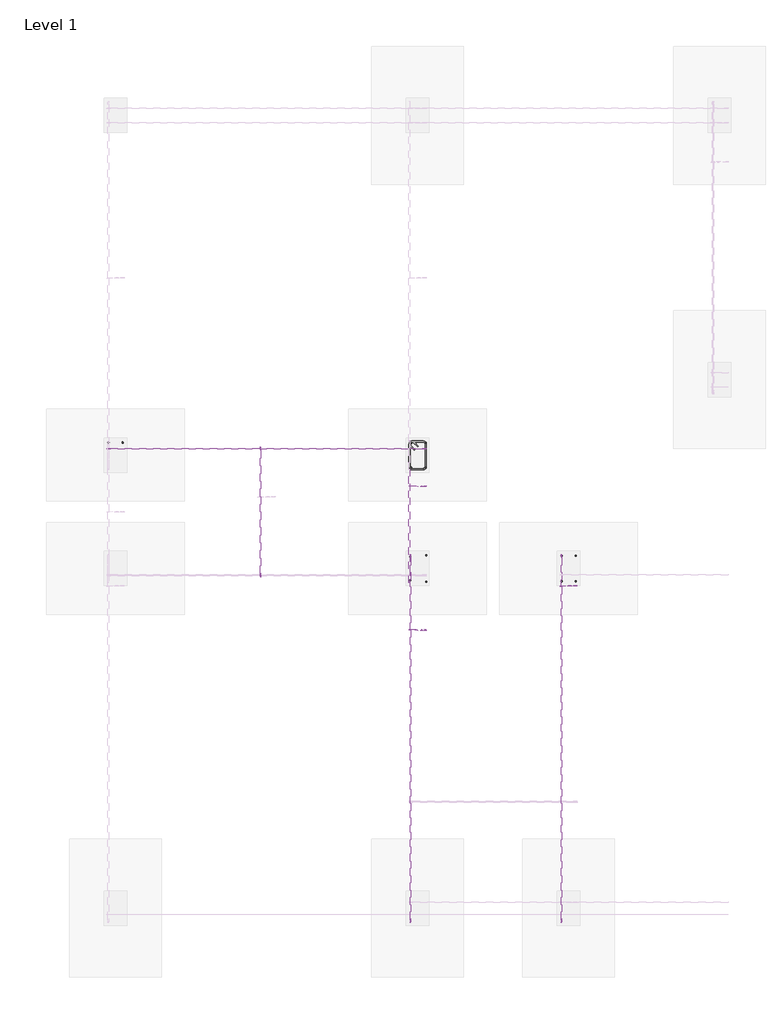
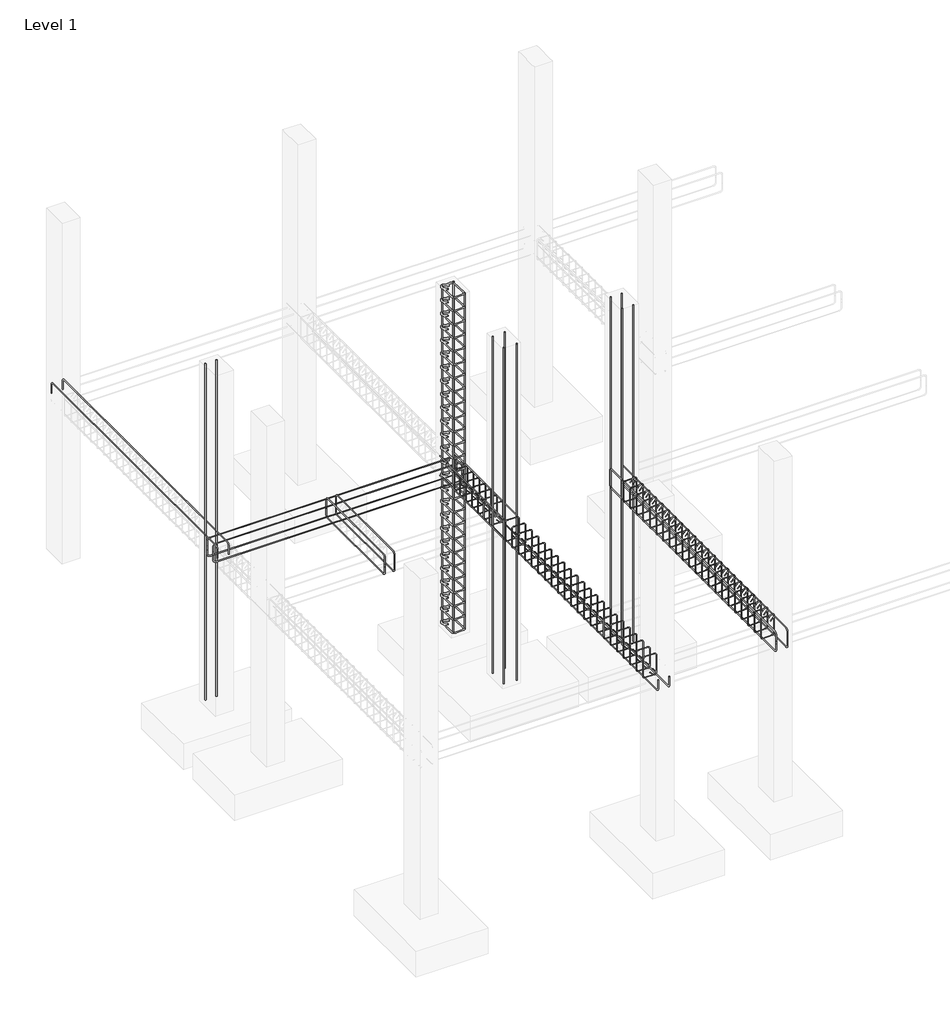
# One storey, part 3 of 5: 21 reinforcing bars.
"""IFC4 building model written with IfcOpenShell, lengths in millimetres."""

from ifc_helpers import new_model, si_unit, point, frame, origin, place, context, project, spatial, polyline, circle_curve, trimmed, segment, composite_curve, source, transform, mapped, element, save
from ifc_brep_helpers import swept_disk

model = new_model("IFC4")

# Units and contexts
model_context = context("Model", 3, world=origin())
ifc_project = project(units=[si_unit("LENGTHUNIT", "METRE", prefix="MILLI")], contexts=[model_context])

# Site, building, storey
site = spatial("IfcSite", under=ifc_project)
building = spatial("IfcBuilding", under=site)
storey = spatial("IfcBuildingStorey", under=building, Name="Level 1", Elevation=0.0)

# Reinforcing bars
placement = place(None, origin())
reinforcing_bar_shape = source(origin(), model_context, "Body", "SolidModel", [
    swept_disk(composite_curve([segment(polyline([(-15212.455746, 8562.3577522, 2793.8967919), (-15212.455746, 8562.3577522, 2946.2967919)]), True, "CONTINUOUS"), segment(trimmed(circle_curve(frame((-15212.455746, 8518.2887522, 2946.2967919), z_axis=(1.0, 0.0, 0.0), x_axis=(0.0, 44.068999999999505, 0.0)), 44.069), [point((-15212.455746, 8562.3577522, 2946.2967919))], [point((-15212.455746, 8518.2887522, 2990.3657919))], True, "CARTESIAN"), True, "CONTINUOUS"), segment(polyline([(-15212.455746, 8518.2887522, 2990.3657919), (-15212.455746, 3737.3647522, 2990.3657919)]), True, "CONTINUOUS"), segment(trimmed(circle_curve(frame((-15212.455746, 3737.3647522, 2946.2967919), z_axis=(1.0, 0.0, 0.0), x_axis=(0.0, 0.0, 44.069000000000415)), 44.069), [point((-15212.455746, 3737.3647522, 2990.3657919))], [point((-15212.455746, 3693.2957522, 2946.2967919))], True, "CARTESIAN"), True, "CONTINUOUS"), segment(polyline([(-15212.455746, 3693.2957522, 2946.2967919), (-15212.455746, 3693.2957522, 2793.8967919)]), True, "CONTINUOUS")], self_intersect=False), 5.969),
])
element("IfcReinforcingBar", 1, at=placement, inside=storey, context=model_context, shape_type="MappedRepresentation", body=[
    mapped(reinforcing_bar_shape, transform((0.0, 0.0, 0.0), x_axis=(1.0, 0.0, 0.0), y_axis=(0.0, 1.0, 0.0), z_axis=(0.0, 0.0, 1.0))),
    mapped(reinforcing_bar_shape, transform((-189.5315837, 0.0, 0.0), x_axis=(1.0, 0.0, 0.0), y_axis=(0.0, 1.0, 0.0), z_axis=(0.0, 0.0, 1.0))),
])
reinforcing_bar_2_shape = source(origin(), model_context, "Body", "SolidModel", [
    swept_disk(composite_curve([segment(polyline([(-15213.892587, 4047.3557031, 38.1), (-15213.892587, 4047.3557031, 6057.9)]), True, "CONTINUOUS")], self_intersect=False), 8.001),
])
element("IfcReinforcingBar", 2, at=placement, inside=storey, context=model_context, shape_type="MappedRepresentation", body=[
    mapped(reinforcing_bar_2_shape, transform((0.0, 0.0, 0.0), x_axis=(1.0, 0.0, 0.0), y_axis=(0.0, 1.0, 0.0), z_axis=(0.0, 0.0, 1.0))),
    mapped(reinforcing_bar_2_shape, transform((-186.6579018, 0.0, 0.0), x_axis=(1.0, 0.0, 0.0), y_axis=(0.0, 1.0, 0.0), z_axis=(0.0, 0.0, 1.0))),
])
reinforcing_bar_3_shape = source(origin(), model_context, "Body", "SolidModel", [
    swept_disk(composite_curve([segment(polyline([(-13226.1955379, 3986.1577522, 2799.588), (-13226.1955379, 3986.1577522, 2951.988)]), True, "CONTINUOUS"), segment(trimmed(circle_curve(frame((-13226.1955379, 3942.0887522, 2951.988), z_axis=(1.0, 0.0, 0.0), x_axis=(0.0, 44.06899999999996, 0.0)), 44.069), [point((-13226.1955379, 3986.1577522, 2951.988))], [point((-13226.1955379, 3942.0887522, 2996.057))], True, "CARTESIAN"), True, "CONTINUOUS"), segment(polyline([(-13226.1955379, 3942.0887522, 2996.057), (-13226.1955379, 2313.5647522, 2996.057)]), True, "CONTINUOUS"), segment(trimmed(circle_curve(frame((-13226.1955379, 2313.5647522, 2951.988), z_axis=(1.0, 0.0, 0.0), x_axis=(0.0, 0.0, 44.06899999999996)), 44.069), [point((-13226.1955379, 2313.5647522, 2996.057))], [point((-13226.1955379, 2269.4957522, 2951.988))], True, "CARTESIAN"), True, "CONTINUOUS"), segment(polyline([(-13226.1955379, 2269.4957522, 2951.988), (-13226.1955379, 2269.4957522, 2799.588)]), True, "CONTINUOUS")], self_intersect=False), 5.969),
])
element("IfcReinforcingBar", 3, at=placement, inside=storey, context=model_context, shape_type="MappedRepresentation", body=[
    mapped(reinforcing_bar_3_shape, transform((0.0, 0.0, 0.0), x_axis=(1.0, 0.0, 0.0), y_axis=(0.0, 1.0, 0.0), z_axis=(0.0, 0.0, 1.0))),
    mapped(reinforcing_bar_3_shape, transform((-162.052, 0.0, 0.0), x_axis=(1.0, 0.0, 0.0), y_axis=(0.0, 1.0, 0.0), z_axis=(0.0, 0.0, 1.0))),
])
reinforcing_bar_4_shape = source(origin(), model_context, "Body", "SolidModel", [
    swept_disk(composite_curve([segment(polyline([(-13388.2475379, 2269.4957522, 2839.212), (-13388.2475379, 2269.4957522, 2686.812)]), True, "CONTINUOUS"), segment(trimmed(circle_curve(frame((-13388.2475379, 2313.5647522, 2686.812), z_axis=(1.0, 0.0, 0.0), x_axis=(0.0, -44.06899999999996, 0.0)), 44.069), [point((-13388.2475379, 2269.4957522, 2686.812))], [point((-13388.2475379, 2313.5647522, 2642.743))], True, "CARTESIAN"), True, "CONTINUOUS"), segment(polyline([(-13388.2475379, 2313.5647522, 2642.743), (-13388.2475379, 3942.0887522, 2642.743)]), True, "CONTINUOUS"), segment(trimmed(circle_curve(frame((-13388.2475379, 3942.0887522, 2686.812), z_axis=(1.0, 0.0, 0.0), x_axis=(0.0, 0.0, -44.06899999999996)), 44.069), [point((-13388.2475379, 3942.0887522, 2642.743))], [point((-13388.2475379, 3986.1577522, 2686.812))], True, "CARTESIAN"), True, "CONTINUOUS"), segment(polyline([(-13388.2475379, 3986.1577522, 2686.812), (-13388.2475379, 3986.1577522, 2839.212)]), True, "CONTINUOUS")], self_intersect=False), 5.969),
])
element("IfcReinforcingBar", 4, at=placement, inside=storey, context=model_context, shape_type="MappedRepresentation", body=[
    mapped(reinforcing_bar_4_shape, transform((0.0, 0.0, 0.0), x_axis=(1.0, 0.0, 0.0), y_axis=(0.0, 1.0, 0.0), z_axis=(0.0, 0.0, 1.0))),
    mapped(reinforcing_bar_4_shape, transform((162.052, 0.0, 0.0), x_axis=(1.0, 0.0, 0.0), y_axis=(0.0, 1.0, 0.0), z_axis=(0.0, 0.0, 1.0))),
])
reinforcing_bar_5_shape = source(origin(), model_context, "Body", "SolidModel", [
    swept_disk(composite_curve([segment(polyline([(-15415.5525379, 3964.464544, 2785.7687919), (-15415.5525379, 3964.464544, 2938.1687919)]), True, "CONTINUOUS"), segment(trimmed(circle_curve(frame((-15371.4835379, 3964.464544, 2938.1687919), z_axis=(0.0, 1.0, 0.0), x_axis=(-44.068999999999505, 0.0, 0.0)), 44.069), [point((-15415.5525379, 3964.464544, 2938.1687919))], [point((-15371.4835379, 3964.464544, 2982.2377919))], True, "CARTESIAN"), True, "CONTINUOUS"), segment(polyline([(-15371.4835379, 3964.464544, 2982.2377919), (-11242.9595379, 3964.464544, 2982.2377919)]), True, "CONTINUOUS"), segment(trimmed(circle_curve(frame((-11242.9595379, 3964.464544, 2938.1687919), z_axis=(0.0, 1.0, 0.0), x_axis=(0.0, 0.0, 44.06899999999996)), 44.069), [point((-11242.9595379, 3964.464544, 2982.2377919))], [point((-11198.8905379, 3964.464544, 2938.1687919))], True, "CARTESIAN"), True, "CONTINUOUS"), segment(polyline([(-11198.8905379, 3964.464544, 2938.1687919), (-11198.8905379, 3964.464544, 2785.7687919)]), True, "CONTINUOUS")], self_intersect=False), 5.969),
])
element("IfcReinforcingBar", 5, at=placement, inside=storey, context=model_context, shape_type="MappedRepresentation", body=[
    mapped(reinforcing_bar_5_shape, transform((0.0, 0.0, 0.0), x_axis=(1.0, 0.0, 0.0), y_axis=(0.0, 1.0, 0.0), z_axis=(0.0, 0.0, 1.0))),
    mapped(reinforcing_bar_5_shape, transform((0.0, -173.2755837, 0.0), x_axis=(1.0, 0.0, 0.0), y_axis=(0.0, 1.0, 0.0), z_axis=(0.0, 0.0, 1.0))),
])
reinforcing_bar_6_shape = source(origin(), model_context, "Body", "SolidModel", [
    swept_disk(composite_curve([segment(polyline([(-11198.8905379, 3964.464544, 2853.0312081), (-11198.8905379, 3964.464544, 2700.6312081)]), True, "CONTINUOUS"), segment(trimmed(circle_curve(frame((-11242.9595379, 3964.464544, 2700.6312081), z_axis=(0.0, 1.0, 0.0), x_axis=(44.068999999999505, 0.0, 0.0)), 44.069), [point((-11198.8905379, 3964.464544, 2700.6312081))], [point((-11242.9595379, 3964.464544, 2656.5622081))], True, "CARTESIAN"), True, "CONTINUOUS"), segment(polyline([(-11242.9595379, 3964.464544, 2656.5622081), (-15371.4835379, 3964.464544, 2656.5622081)]), True, "CONTINUOUS"), segment(trimmed(circle_curve(frame((-15371.4835379, 3964.464544, 2700.6312081), z_axis=(0.0, 1.0, 0.0), x_axis=(0.0, 0.0, -44.06899999999996)), 44.069), [point((-15371.4835379, 3964.464544, 2656.5622081))], [point((-15415.5525379, 3964.464544, 2700.6312081))], True, "CARTESIAN"), True, "CONTINUOUS"), segment(polyline([(-15415.5525379, 3964.464544, 2700.6312081), (-15415.5525379, 3964.464544, 2853.0312081)]), True, "CONTINUOUS")], self_intersect=False), 5.969),
])
element("IfcReinforcingBar", 6, at=placement, inside=storey, context=model_context, shape_type="MappedRepresentation", body=[
    mapped(reinforcing_bar_6_shape, transform((0.0, 0.0, 0.0), x_axis=(1.0, 0.0, 0.0), y_axis=(0.0, 1.0, 0.0), z_axis=(0.0, 0.0, 1.0))),
    mapped(reinforcing_bar_6_shape, transform((0.0, -173.2755837, 0.0), x_axis=(1.0, 0.0, 0.0), y_axis=(0.0, 1.0, 0.0), z_axis=(0.0, 0.0, 1.0))),
])
reinforcing_bar_7_shape = source(origin(), model_context, "Body", "SolidModel", [
    swept_disk(composite_curve([segment(polyline([(-11392.4224888, 4039.2277031, 38.1), (-11392.4224888, 4039.2277031, 6057.9)]), True, "CONTINUOUS")], self_intersect=False), 8.001),
])
element("IfcReinforcingBar", 7, at=placement, inside=storey, context=model_context, shape_type="MappedRepresentation", body=[
    mapped(reinforcing_bar_7_shape, transform((0.0, 0.0, 0.0), x_axis=(1.0, 0.0, 0.0), y_axis=(0.0, 1.0, 0.0), z_axis=(0.0, 0.0, 1.0))),
    mapped(reinforcing_bar_7_shape, transform((0.0, -322.8019018, 0.0), x_axis=(1.0, 0.0, 0.0), y_axis=(0.0, 1.0, 0.0), z_axis=(0.0, 0.0, 1.0))),
])
reinforcing_bar_8_shape = source(origin(), model_context, "Body", "SolidModel", [
    swept_disk(composite_curve([segment(polyline([(-11200.9225379, 4044.3237522, 6057.9), (-11200.9225379, 4044.3237522, 38.1)]), True, "CONTINUOUS")], self_intersect=False), 8.001),
])
element("IfcReinforcingBar", 8, at=placement, inside=storey, context=model_context, shape_type="MappedRepresentation", body=[
    mapped(reinforcing_bar_8_shape, transform((0.0, 0.0, 0.0), x_axis=(1.0, 0.0, 0.0), y_axis=(0.0, 1.0, 0.0), z_axis=(0.0, 0.0, 1.0))),
    mapped(reinforcing_bar_8_shape, transform((0.0, -332.994, 0.0), x_axis=(1.0, 0.0, 0.0), y_axis=(0.0, 1.0, 0.0), z_axis=(0.0, 0.0, 1.0))),
])
reinforcing_bar_9_shape = source(origin(), model_context, "Body", "SolidModel", [
    swept_disk(composite_curve([segment(polyline([(-11301.6364658, 3995.6778273, 46.101), (-11356.5014643, 4050.5428258, 46.101)]), True, "CONTINUOUS"), segment(trimmed(circle_curve(frame((-11380.1195379, 4026.9247522, 46.101), z_axis=(0.0, 0.0, 1.0), x_axis=(23.61807360000057, 23.618073600000116, 0.0)), 33.401), [point((-11356.5014643, 4050.5428258, 46.101))], [point((-11413.5205379, 4026.9247522, 46.101))], True, "CARTESIAN"), True, "CONTINUOUS"), segment(polyline([(-11413.5205379, 4026.9247522, 46.101), (-11413.5205379, 3728.7287522, 46.101)]), True, "CONTINUOUS"), segment(trimmed(circle_curve(frame((-11380.1195379, 3728.7287522, 46.101), z_axis=(0.0, 0.0, 1.0), x_axis=(-33.40099999999984, 0.0, 0.0)), 33.401), [point((-11413.5205379, 3728.7287522, 46.101))], [point((-11380.1195379, 3695.3277522, 46.101))], True, "CARTESIAN"), True, "CONTINUOUS"), segment(polyline([(-11380.1195379, 3695.3277522, 46.101), (-11234.3235379, 3695.3277522, 46.101)]), True, "CONTINUOUS"), segment(trimmed(circle_curve(frame((-11234.3235379, 3728.696699, 44.6380608), z_axis=(0.0, 0.043799263856762964, 0.9990403517804503), x_axis=(0.0, -33.36894680000023, 1.462939200000001)), 33.401), [point((-11234.3235379, 3695.3277522, 46.101))], [point((-11200.9225379, 3728.696699, 44.6380608))], True, "CARTESIAN"), True, "CONTINUOUS"), segment(polyline([(-11200.9225379, 3728.696699, 44.6380608), (-11200.9225379, 4026.9568054, 31.5619392)]), True, "CONTINUOUS"), segment(trimmed(circle_curve(frame((-11234.3235379, 4026.9568054, 31.5619392), z_axis=(0.0, 0.043799263856762964, 0.9990403517804503), x_axis=(33.40099999999984, 0.0, 0.0)), 33.401), [point((-11200.9225379, 4026.9568054, 31.5619392))], [point((-11234.3235379, 4060.3257522, 30.099))], True, "CARTESIAN"), True, "CONTINUOUS"), segment(polyline([(-11234.3235379, 4060.3257522, 30.099), (-11380.1195379, 4060.3257522, 30.099)]), True, "CONTINUOUS"), segment(trimmed(circle_curve(frame((-11380.1195379, 4026.9247522, 30.099), z_axis=(0.0, 0.0, 1.0), x_axis=(0.0, 33.40099999999984, 0.0)), 33.401), [point((-11380.1195379, 4060.3257522, 30.099))], [point((-11403.7376115, 4003.3066786, 30.099))], True, "CARTESIAN"), True, "CONTINUOUS"), segment(polyline([(-11403.7376115, 4003.3066786, 30.099), (-11348.872613, 3948.4416801, 30.099)]), True, "CONTINUOUS")], self_intersect=False), 8.001),
])
element("IfcReinforcingBar", 9, at=placement, inside=storey, context=model_context, shape_type="MappedRepresentation", body=[
    mapped(reinforcing_bar_9_shape, transform((0.0, 0.0, 0.0), x_axis=(1.0, 0.0, 0.0), y_axis=(0.0, 1.0, 0.0), z_axis=(0.0, 0.0, 1.0))),
    mapped(reinforcing_bar_9_shape, transform((0.0, 0.0, 240.15192), x_axis=(1.0, 0.0, 0.0), y_axis=(0.0, 1.0, 0.0), z_axis=(0.0, 0.0, 1.0))),
    mapped(reinforcing_bar_9_shape, transform((0.0, 0.0, 480.30384), x_axis=(1.0, 0.0, 0.0), y_axis=(0.0, 1.0, 0.0), z_axis=(0.0, 0.0, 1.0))),
    mapped(reinforcing_bar_9_shape, transform((0.0, 0.0, 720.45576), x_axis=(1.0, 0.0, 0.0), y_axis=(0.0, 1.0, 0.0), z_axis=(0.0, 0.0, 1.0))),
    mapped(reinforcing_bar_9_shape, transform((0.0, 0.0, 960.60768), x_axis=(1.0, 0.0, 0.0), y_axis=(0.0, 1.0, 0.0), z_axis=(0.0, 0.0, 1.0))),
    mapped(reinforcing_bar_9_shape, transform((0.0, 0.0, 1200.7596), x_axis=(1.0, 0.0, 0.0), y_axis=(0.0, 1.0, 0.0), z_axis=(0.0, 0.0, 1.0))),
    mapped(reinforcing_bar_9_shape, transform((0.0, 0.0, 1440.91152), x_axis=(1.0, 0.0, 0.0), y_axis=(0.0, 1.0, 0.0), z_axis=(0.0, 0.0, 1.0))),
    mapped(reinforcing_bar_9_shape, transform((0.0, 0.0, 1681.06344), x_axis=(1.0, 0.0, 0.0), y_axis=(0.0, 1.0, 0.0), z_axis=(0.0, 0.0, 1.0))),
    mapped(reinforcing_bar_9_shape, transform((0.0, 0.0, 1921.21536), x_axis=(1.0, 0.0, 0.0), y_axis=(0.0, 1.0, 0.0), z_axis=(0.0, 0.0, 1.0))),
    mapped(reinforcing_bar_9_shape, transform((0.0, 0.0, 2161.36728), x_axis=(1.0, 0.0, 0.0), y_axis=(0.0, 1.0, 0.0), z_axis=(0.0, 0.0, 1.0))),
    mapped(reinforcing_bar_9_shape, transform((0.0, 0.0, 2401.5192), x_axis=(1.0, 0.0, 0.0), y_axis=(0.0, 1.0, 0.0), z_axis=(0.0, 0.0, 1.0))),
    mapped(reinforcing_bar_9_shape, transform((0.0, 0.0, 2641.67112), x_axis=(1.0, 0.0, 0.0), y_axis=(0.0, 1.0, 0.0), z_axis=(0.0, 0.0, 1.0))),
    mapped(reinforcing_bar_9_shape, transform((0.0, 0.0, 2881.82304), x_axis=(1.0, 0.0, 0.0), y_axis=(0.0, 1.0, 0.0), z_axis=(0.0, 0.0, 1.0))),
    mapped(reinforcing_bar_9_shape, transform((0.0, 0.0, 3121.97496), x_axis=(1.0, 0.0, 0.0), y_axis=(0.0, 1.0, 0.0), z_axis=(0.0, 0.0, 1.0))),
    mapped(reinforcing_bar_9_shape, transform((0.0, 0.0, 3362.12688), x_axis=(1.0, 0.0, 0.0), y_axis=(0.0, 1.0, 0.0), z_axis=(0.0, 0.0, 1.0))),
    mapped(reinforcing_bar_9_shape, transform((0.0, 0.0, 3602.2788), x_axis=(1.0, 0.0, 0.0), y_axis=(0.0, 1.0, 0.0), z_axis=(0.0, 0.0, 1.0))),
    mapped(reinforcing_bar_9_shape, transform((0.0, 0.0, 3842.43072), x_axis=(1.0, 0.0, 0.0), y_axis=(0.0, 1.0, 0.0), z_axis=(0.0, 0.0, 1.0))),
    mapped(reinforcing_bar_9_shape, transform((0.0, 0.0, 4082.58264), x_axis=(1.0, 0.0, 0.0), y_axis=(0.0, 1.0, 0.0), z_axis=(0.0, 0.0, 1.0))),
    mapped(reinforcing_bar_9_shape, transform((0.0, 0.0, 4322.73456), x_axis=(1.0, 0.0, 0.0), y_axis=(0.0, 1.0, 0.0), z_axis=(0.0, 0.0, 1.0))),
    mapped(reinforcing_bar_9_shape, transform((0.0, 0.0, 4562.88648), x_axis=(1.0, 0.0, 0.0), y_axis=(0.0, 1.0, 0.0), z_axis=(0.0, 0.0, 1.0))),
    mapped(reinforcing_bar_9_shape, transform((0.0, 0.0, 4803.0384), x_axis=(1.0, 0.0, 0.0), y_axis=(0.0, 1.0, 0.0), z_axis=(0.0, 0.0, 1.0))),
    mapped(reinforcing_bar_9_shape, transform((0.0, 0.0, 5043.19032), x_axis=(1.0, 0.0, 0.0), y_axis=(0.0, 1.0, 0.0), z_axis=(0.0, 0.0, 1.0))),
    mapped(reinforcing_bar_9_shape, transform((0.0, 0.0, 5283.34224), x_axis=(1.0, 0.0, 0.0), y_axis=(0.0, 1.0, 0.0), z_axis=(0.0, 0.0, 1.0))),
    mapped(reinforcing_bar_9_shape, transform((0.0, 0.0, 5523.49416), x_axis=(1.0, 0.0, 0.0), y_axis=(0.0, 1.0, 0.0), z_axis=(0.0, 0.0, 1.0))),
    mapped(reinforcing_bar_9_shape, transform((0.0, 0.0, 5763.64608), x_axis=(1.0, 0.0, 0.0), y_axis=(0.0, 1.0, 0.0), z_axis=(0.0, 0.0, 1.0))),
    mapped(reinforcing_bar_9_shape, transform((0.0, 0.0, 6003.798), x_axis=(1.0, 0.0, 0.0), y_axis=(0.0, 1.0, 0.0), z_axis=(0.0, 0.0, 1.0))),
])
reinforcing_bar_10_shape = source(origin(), model_context, "Body", "SolidModel", [
    swept_disk(composite_curve([segment(polyline([(-11192.9215379, 2203.2017522, 38.1), (-11192.9215379, 2203.2017522, 6057.9)]), True, "CONTINUOUS")], self_intersect=False), 8.001),
])
element("IfcReinforcingBar", 10, at=placement, inside=storey, context=model_context, shape_type="MappedRepresentation", body=[
    mapped(reinforcing_bar_10_shape, transform((0.0, 0.0, 0.0), x_axis=(1.0, 0.0, 0.0), y_axis=(0.0, 1.0, 0.0), z_axis=(0.0, 0.0, 1.0))),
    mapped(reinforcing_bar_10_shape, transform((0.0, 349.25, 0.0), x_axis=(1.0, 0.0, 0.0), y_axis=(0.0, 1.0, 0.0), z_axis=(0.0, 0.0, 1.0))),
])
reinforcing_bar_11_shape = source(origin(), model_context, "Body", "SolidModel", [
    swept_disk(composite_curve([segment(polyline([(-11405.6465379, 2535.0527522, 6057.9), (-11405.6465379, 2535.0527522, 38.1)]), True, "CONTINUOUS")], self_intersect=False), 8.001),
])
element("IfcReinforcingBar", 11, at=placement, inside=storey, context=model_context, shape_type="MappedRepresentation", body=[
    mapped(reinforcing_bar_11_shape, transform((0.0, 0.0, 0.0), x_axis=(1.0, 0.0, 0.0), y_axis=(0.0, 1.0, 0.0), z_axis=(0.0, 0.0, 1.0))),
    mapped(reinforcing_bar_11_shape, transform((0.0, -314.452, 0.0), x_axis=(1.0, 0.0, 0.0), y_axis=(0.0, 1.0, 0.0), z_axis=(0.0, 0.0, 1.0))),
])
reinforcing_bar_12_shape = source(origin(), model_context, "Body", "SolidModel", [
    swept_disk(composite_curve([segment(polyline([(-11198.8905379, 4068.3267522, 2996.057), (-11198.8905379, 2187.3267522, 2996.057)]), True, "CONTINUOUS")], self_intersect=False), 5.969),
])
element("IfcReinforcingBar", 12, at=placement, inside=storey, context=model_context, shape_type="MappedRepresentation", body=[
    mapped(reinforcing_bar_12_shape, transform((0.0, 0.0, 0.0), x_axis=(1.0, 0.0, 0.0), y_axis=(0.0, 1.0, 0.0), z_axis=(0.0, 0.0, 1.0))),
    mapped(reinforcing_bar_12_shape, transform((-216.662, 0.0, 0.0), x_axis=(1.0, 0.0, 0.0), y_axis=(0.0, 1.0, 0.0), z_axis=(0.0, 0.0, 1.0))),
])
reinforcing_bar_13_shape = source(origin(), model_context, "Body", "SolidModel", [
    swept_disk(composite_curve([segment(polyline([(-11212.455746, 2187.3267522, 2648.4342081), (-11212.455746, 4068.3267522, 2648.4342081)]), True, "CONTINUOUS")], self_intersect=False), 5.969),
])
element("IfcReinforcingBar", 13, at=placement, inside=storey, context=model_context, shape_type="MappedRepresentation", body=[
    mapped(reinforcing_bar_13_shape, transform((0.0, 0.0, 0.0), x_axis=(1.0, 0.0, 0.0), y_axis=(0.0, 1.0, 0.0), z_axis=(0.0, 0.0, 1.0))),
    mapped(reinforcing_bar_13_shape, transform((-203.0967919, 0.0, 0.0), x_axis=(1.0, 0.0, 0.0), y_axis=(0.0, 1.0, 0.0), z_axis=(0.0, 0.0, 1.0))),
])
reinforcing_bar_14_shape = source(origin(), model_context, "Body", "SolidModel", [
    swept_disk(composite_curve([segment(polyline([(-11212.455746, -2306.7042478, 2844.9032081), (-11212.455746, -2306.7042478, 2692.5032081)]), True, "CONTINUOUS"), segment(trimmed(circle_curve(frame((-11212.455746, -2262.6352478, 2692.5032081), z_axis=(1.0, 0.0, 0.0), x_axis=(0.0, -44.06899999999996, 0.0)), 44.069), [point((-11212.455746, -2306.7042478, 2692.5032081))], [point((-11212.455746, -2262.6352478, 2648.4342081))], True, "CARTESIAN"), True, "CONTINUOUS"), segment(polyline([(-11212.455746, -2262.6352478, 2648.4342081), (-11212.455746, 2518.2887522, 2648.4342081)]), True, "CONTINUOUS"), segment(trimmed(circle_curve(frame((-11212.455746, 2518.2887522, 2692.5032081), z_axis=(1.0, 0.0, 0.0), x_axis=(0.0, 0.0, -44.06899999999996)), 44.069), [point((-11212.455746, 2518.2887522, 2648.4342081))], [point((-11212.455746, 2562.3577522, 2692.5032081))], True, "CARTESIAN"), True, "CONTINUOUS"), segment(polyline([(-11212.455746, 2562.3577522, 2692.5032081), (-11212.455746, 2562.3577522, 2844.9032081)]), True, "CONTINUOUS")], self_intersect=False), 5.969),
])
element("IfcReinforcingBar", 14, at=placement, inside=storey, context=model_context, shape_type="MappedRepresentation", body=[
    mapped(reinforcing_bar_14_shape, transform((0.0, 0.0, 0.0), x_axis=(1.0, 0.0, 0.0), y_axis=(0.0, 1.0, 0.0), z_axis=(0.0, 0.0, 1.0))),
    mapped(reinforcing_bar_14_shape, transform((-189.5315837, 0.0, 0.0), x_axis=(1.0, 0.0, 0.0), y_axis=(0.0, 1.0, 0.0), z_axis=(0.0, 0.0, 1.0))),
])
reinforcing_bar_15_shape = source(origin(), model_context, "Body", "SolidModel", [
    swept_disk(composite_curve([segment(polyline([(-11260.3161447, -1889.6362478, 2737.7833901), (-11205.4511463, -1889.6362478, 2682.9183916)]), True, "CONTINUOUS"), segment(trimmed(circle_curve(frame((-11226.1955379, -1889.6362478, 2662.174), z_axis=(0.0, 1.0, 0.0), x_axis=(20.74439159999929, 0.0, 20.7443916000002)), 29.337), [point((-11205.4511463, -1889.6362478, 2682.9183916))], [point((-11226.1955379, -1889.6362478, 2632.837))], True, "CARTESIAN"), True, "CONTINUOUS"), segment(polyline([(-11226.1955379, -1889.6362478, 2632.837), (-11388.2475379, -1889.6362478, 2632.837)]), True, "CONTINUOUS"), segment(trimmed(circle_curve(frame((-11388.2475379, -1889.6362478, 2662.174), z_axis=(0.0, 1.0, 0.0), x_axis=(0.0, 0.0, -29.33699999999999)), 29.337), [point((-11388.2475379, -1889.6362478, 2632.837))], [point((-11417.5845379, -1889.6362478, 2662.174))], True, "CARTESIAN"), True, "CONTINUOUS"), segment(polyline([(-11417.5845379, -1889.6362478, 2662.174), (-11417.5845379, -1889.6362478, 2976.626)]), True, "CONTINUOUS"), segment(trimmed(circle_curve(frame((-11388.2661869, -1890.6821269, 2976.626), z_axis=(0.03565051078635425, 0.9993643184948481, 0.0), x_axis=(-29.318350999999893, 1.0458790999998655, 0.0)), 29.337), [point((-11417.5845379, -1889.6362478, 2976.626))], [point((-11388.2661869, -1890.6821269, 3005.963))], True, "CARTESIAN"), True, "CONTINUOUS"), segment(polyline([(-11388.2661869, -1890.6821269, 3005.963), (-11226.1768889, -1896.4643688, 3005.963)]), True, "CONTINUOUS"), segment(trimmed(circle_curve(frame((-11226.1768889, -1896.4643688, 2976.626), z_axis=(0.03565051078635425, 0.9993643184948481, 0.0), x_axis=(0.0, 0.0, 29.33699999999999)), 29.337), [point((-11226.1768889, -1896.4643688, 3005.963))], [point((-11196.8585379, -1897.5102478, 2976.626))], True, "CARTESIAN"), True, "CONTINUOUS"), segment(polyline([(-11196.8585379, -1897.5102478, 2976.626), (-11196.8585379, -1897.5102478, 2662.174)]), True, "CONTINUOUS"), segment(trimmed(circle_curve(frame((-11226.1955379, -1897.5102478, 2662.174), z_axis=(0.0, 1.0, 0.0), x_axis=(29.336999999999534, 0.0, 0.0)), 29.337), [point((-11196.8585379, -1897.5102478, 2662.174))], [point((-11246.9399295, -1897.5102478, 2641.4296084))], True, "CARTESIAN"), True, "CONTINUOUS"), segment(polyline([(-11246.9399295, -1897.5102478, 2641.4296084), (-11301.804928, -1897.5102478, 2696.2946068)]), True, "CONTINUOUS")], self_intersect=False), 3.937),
])
element("IfcReinforcingBar", 15, at=placement, inside=storey, context=model_context, shape_type="MappedRepresentation", body=[
    mapped(reinforcing_bar_15_shape, transform((0.0, 0.0, 0.0), x_axis=(1.0, 0.0, 0.0), y_axis=(0.0, 1.0, 0.0), z_axis=(0.0, 0.0, 1.0))),
    mapped(reinforcing_bar_15_shape, transform((0.0, 192.1393333, 0.0), x_axis=(1.0, 0.0, 0.0), y_axis=(0.0, 1.0, 0.0), z_axis=(0.0, 0.0, 1.0))),
    mapped(reinforcing_bar_15_shape, transform((0.0, 384.2786667, 0.0), x_axis=(1.0, 0.0, 0.0), y_axis=(0.0, 1.0, 0.0), z_axis=(0.0, 0.0, 1.0))),
    mapped(reinforcing_bar_15_shape, transform((0.0, 576.418, 0.0), x_axis=(1.0, 0.0, 0.0), y_axis=(0.0, 1.0, 0.0), z_axis=(0.0, 0.0, 1.0))),
    mapped(reinforcing_bar_15_shape, transform((0.0, 768.5573333, 0.0), x_axis=(1.0, 0.0, 0.0), y_axis=(0.0, 1.0, 0.0), z_axis=(0.0, 0.0, 1.0))),
    mapped(reinforcing_bar_15_shape, transform((0.0, 960.6966667, 0.0), x_axis=(1.0, 0.0, 0.0), y_axis=(0.0, 1.0, 0.0), z_axis=(0.0, 0.0, 1.0))),
    mapped(reinforcing_bar_15_shape, transform((0.0, 1152.836, 0.0), x_axis=(1.0, 0.0, 0.0), y_axis=(0.0, 1.0, 0.0), z_axis=(0.0, 0.0, 1.0))),
    mapped(reinforcing_bar_15_shape, transform((0.0, 1344.9753333, 0.0), x_axis=(1.0, 0.0, 0.0), y_axis=(0.0, 1.0, 0.0), z_axis=(0.0, 0.0, 1.0))),
    mapped(reinforcing_bar_15_shape, transform((0.0, 1537.1146667, 0.0), x_axis=(1.0, 0.0, 0.0), y_axis=(0.0, 1.0, 0.0), z_axis=(0.0, 0.0, 1.0))),
    mapped(reinforcing_bar_15_shape, transform((0.0, 1729.254, 0.0), x_axis=(1.0, 0.0, 0.0), y_axis=(0.0, 1.0, 0.0), z_axis=(0.0, 0.0, 1.0))),
    mapped(reinforcing_bar_15_shape, transform((0.0, 1921.3933333, 0.0), x_axis=(1.0, 0.0, 0.0), y_axis=(0.0, 1.0, 0.0), z_axis=(0.0, 0.0, 1.0))),
    mapped(reinforcing_bar_15_shape, transform((0.0, 2113.5326667, 0.0), x_axis=(1.0, 0.0, 0.0), y_axis=(0.0, 1.0, 0.0), z_axis=(0.0, 0.0, 1.0))),
    mapped(reinforcing_bar_15_shape, transform((0.0, 2305.672, 0.0), x_axis=(1.0, 0.0, 0.0), y_axis=(0.0, 1.0, 0.0), z_axis=(0.0, 0.0, 1.0))),
    mapped(reinforcing_bar_15_shape, transform((0.0, 2497.8113333, 0.0), x_axis=(1.0, 0.0, 0.0), y_axis=(0.0, 1.0, 0.0), z_axis=(0.0, 0.0, 1.0))),
    mapped(reinforcing_bar_15_shape, transform((0.0, 2689.9506667, 0.0), x_axis=(1.0, 0.0, 0.0), y_axis=(0.0, 1.0, 0.0), z_axis=(0.0, 0.0, 1.0))),
    mapped(reinforcing_bar_15_shape, transform((0.0, 2882.09, 0.0), x_axis=(1.0, 0.0, 0.0), y_axis=(0.0, 1.0, 0.0), z_axis=(0.0, 0.0, 1.0))),
    mapped(reinforcing_bar_15_shape, transform((0.0, 3074.2293333, 0.0), x_axis=(1.0, 0.0, 0.0), y_axis=(0.0, 1.0, 0.0), z_axis=(0.0, 0.0, 1.0))),
    mapped(reinforcing_bar_15_shape, transform((0.0, 3266.3686667, 0.0), x_axis=(1.0, 0.0, 0.0), y_axis=(0.0, 1.0, 0.0), z_axis=(0.0, 0.0, 1.0))),
    mapped(reinforcing_bar_15_shape, transform((0.0, 3458.508, 0.0), x_axis=(1.0, 0.0, 0.0), y_axis=(0.0, 1.0, 0.0), z_axis=(0.0, 0.0, 1.0))),
    mapped(reinforcing_bar_15_shape, transform((0.0, 3650.6473333, 0.0), x_axis=(1.0, 0.0, 0.0), y_axis=(0.0, 1.0, 0.0), z_axis=(0.0, 0.0, 1.0))),
    mapped(reinforcing_bar_15_shape, transform((0.0, 3842.7866667, 0.0), x_axis=(1.0, 0.0, 0.0), y_axis=(0.0, 1.0, 0.0), z_axis=(0.0, 0.0, 1.0))),
    mapped(reinforcing_bar_15_shape, transform((0.0, 4034.926, 0.0), x_axis=(1.0, 0.0, 0.0), y_axis=(0.0, 1.0, 0.0), z_axis=(0.0, 0.0, 1.0))),
])
reinforcing_bar_16_shape = source(origin(), model_context, "Body", "SolidModel", [
    swept_disk(composite_curve([segment(polyline([(-11260.3161447, 2610.3637522, 2737.7833901), (-11205.4511463, 2610.3637522, 2682.9183916)]), True, "CONTINUOUS"), segment(trimmed(circle_curve(frame((-11226.1955379, 2610.3637522, 2662.174), z_axis=(0.0, 1.0, 0.0), x_axis=(20.74439159999929, 0.0, 20.7443916000002)), 29.337), [point((-11205.4511463, 2610.3637522, 2682.9183916))], [point((-11226.1955379, 2610.3637522, 2632.837))], True, "CARTESIAN"), True, "CONTINUOUS"), segment(polyline([(-11226.1955379, 2610.3637522, 2632.837), (-11388.2475379, 2610.3637522, 2632.837)]), True, "CONTINUOUS"), segment(trimmed(circle_curve(frame((-11388.2475379, 2610.3637522, 2662.174), z_axis=(0.0, 1.0, 0.0), x_axis=(0.0, 0.0, -29.33699999999999)), 29.337), [point((-11388.2475379, 2610.3637522, 2632.837))], [point((-11417.5845379, 2610.3637522, 2662.174))], True, "CARTESIAN"), True, "CONTINUOUS"), segment(polyline([(-11417.5845379, 2610.3637522, 2662.174), (-11417.5845379, 2610.3637522, 2976.626)]), True, "CONTINUOUS"), segment(trimmed(circle_curve(frame((-11388.2661869, 2609.3178731, 2976.626), z_axis=(0.03565051078635292, 0.9993643184948482, 0.0), x_axis=(-29.318350999999893, 1.0458791000000929, 0.0)), 29.337), [point((-11417.5845379, 2610.3637522, 2976.626))], [point((-11388.2661869, 2609.3178731, 3005.963))], True, "CARTESIAN"), True, "CONTINUOUS"), segment(polyline([(-11388.2661869, 2609.3178731, 3005.963), (-11226.1768889, 2603.5356312, 3005.963)]), True, "CONTINUOUS"), segment(trimmed(circle_curve(frame((-11226.1768889, 2603.5356312, 2976.626), z_axis=(0.03565051078635292, 0.9993643184948482, 0.0), x_axis=(0.0, 0.0, 29.33699999999999)), 29.337), [point((-11226.1768889, 2603.5356312, 3005.963))], [point((-11196.8585379, 2602.4897522, 2976.626))], True, "CARTESIAN"), True, "CONTINUOUS"), segment(polyline([(-11196.8585379, 2602.4897522, 2976.626), (-11196.8585379, 2602.4897522, 2662.174)]), True, "CONTINUOUS"), segment(trimmed(circle_curve(frame((-11226.1955379, 2602.4897522, 2662.174), z_axis=(0.0, 1.0, 0.0), x_axis=(29.336999999999534, 0.0, 0.0)), 29.337), [point((-11196.8585379, 2602.4897522, 2662.174))], [point((-11246.9399295, 2602.4897522, 2641.4296084))], True, "CARTESIAN"), True, "CONTINUOUS"), segment(polyline([(-11246.9399295, 2602.4897522, 2641.4296084), (-11301.804928, 2602.4897522, 2696.2946068)]), True, "CONTINUOUS")], self_intersect=False), 3.937),
])
element("IfcReinforcingBar", 16, at=placement, inside=storey, context=model_context, shape_type="MappedRepresentation", body=[
    mapped(reinforcing_bar_16_shape, transform((0.0, 0.0, 0.0), x_axis=(1.0, 0.0, 0.0), y_axis=(0.0, 1.0, 0.0), z_axis=(0.0, 0.0, 1.0))),
    mapped(reinforcing_bar_16_shape, transform((0.0, 172.4876667, 0.0), x_axis=(1.0, 0.0, 0.0), y_axis=(0.0, 1.0, 0.0), z_axis=(0.0, 0.0, 1.0))),
    mapped(reinforcing_bar_16_shape, transform((0.0, 344.9753333, 0.0), x_axis=(1.0, 0.0, 0.0), y_axis=(0.0, 1.0, 0.0), z_axis=(0.0, 0.0, 1.0))),
    mapped(reinforcing_bar_16_shape, transform((0.0, 517.463, 0.0), x_axis=(1.0, 0.0, 0.0), y_axis=(0.0, 1.0, 0.0), z_axis=(0.0, 0.0, 1.0))),
    mapped(reinforcing_bar_16_shape, transform((0.0, 689.9506667, 0.0), x_axis=(1.0, 0.0, 0.0), y_axis=(0.0, 1.0, 0.0), z_axis=(0.0, 0.0, 1.0))),
    mapped(reinforcing_bar_16_shape, transform((0.0, 862.4383333, 0.0), x_axis=(1.0, 0.0, 0.0), y_axis=(0.0, 1.0, 0.0), z_axis=(0.0, 0.0, 1.0))),
    mapped(reinforcing_bar_16_shape, transform((0.0, 1034.926, 0.0), x_axis=(1.0, 0.0, 0.0), y_axis=(0.0, 1.0, 0.0), z_axis=(0.0, 0.0, 1.0))),
])
reinforcing_bar_17_shape = source(origin(), model_context, "Body", "SolidModel", [
    swept_disk(composite_curve([segment(polyline([(-9213.892587, 2547.3557031, 38.1), (-9213.892587, 2547.3557031, 6057.9)]), True, "CONTINUOUS")], self_intersect=False), 8.001),
])
element("IfcReinforcingBar", 17, at=placement, inside=storey, context=model_context, shape_type="MappedRepresentation", body=[
    mapped(reinforcing_bar_17_shape, transform((0.0, 0.0, 0.0), x_axis=(1.0, 0.0, 0.0), y_axis=(0.0, 1.0, 0.0), z_axis=(0.0, 0.0, 1.0))),
    mapped(reinforcing_bar_17_shape, transform((-186.6579018, 0.0, 0.0), x_axis=(1.0, 0.0, 0.0), y_axis=(0.0, 1.0, 0.0), z_axis=(0.0, 0.0, 1.0))),
])
reinforcing_bar_18_shape = source(origin(), model_context, "Body", "SolidModel", [
    swept_disk(composite_curve([segment(polyline([(-9213.892587, 2208.2978013, 6057.9), (-9213.892587, 2208.2978013, 38.1)]), True, "CONTINUOUS")], self_intersect=False), 8.001),
])
element("IfcReinforcingBar", 18, at=placement, inside=storey, context=model_context, shape_type="MappedRepresentation", body=[
    mapped(reinforcing_bar_18_shape, transform((0.0, 0.0, 0.0), x_axis=(1.0, 0.0, 0.0), y_axis=(0.0, 1.0, 0.0), z_axis=(0.0, 0.0, 1.0))),
    mapped(reinforcing_bar_18_shape, transform((-186.6579018, 0.0, 0.0), x_axis=(1.0, 0.0, 0.0), y_axis=(0.0, 1.0, 0.0), z_axis=(0.0, 0.0, 1.0))),
])
reinforcing_bar_19_shape = source(origin(), model_context, "Body", "SolidModel", [
    swept_disk(composite_curve([segment(polyline([(-9212.455746, 2562.3577522, 2793.8967919), (-9212.455746, 2562.3577522, 2946.2967919)]), True, "CONTINUOUS"), segment(trimmed(circle_curve(frame((-9212.455746, 2518.2887522, 2946.2967919), z_axis=(1.0, 0.0, 0.0), x_axis=(0.0, 44.06899999999996, 0.0)), 44.069), [point((-9212.455746, 2562.3577522, 2946.2967919))], [point((-9212.455746, 2518.2887522, 2990.3657919))], True, "CARTESIAN"), True, "CONTINUOUS"), segment(polyline([(-9212.455746, 2518.2887522, 2990.3657919), (-9212.455746, -2262.6352478, 2990.3657919)]), True, "CONTINUOUS"), segment(trimmed(circle_curve(frame((-9212.455746, -2262.6352478, 2946.2967919), z_axis=(1.0, 0.0, 0.0), x_axis=(0.0, 0.0, 44.069000000000415)), 44.069), [point((-9212.455746, -2262.6352478, 2990.3657919))], [point((-9212.455746, -2306.7042478, 2946.2967919))], True, "CARTESIAN"), True, "CONTINUOUS"), segment(polyline([(-9212.455746, -2306.7042478, 2946.2967919), (-9212.455746, -2306.7042478, 2793.8967919)]), True, "CONTINUOUS")], self_intersect=False), 5.969),
])
element("IfcReinforcingBar", 19, at=placement, inside=storey, context=model_context, shape_type="MappedRepresentation", body=[
    mapped(reinforcing_bar_19_shape, transform((0.0, 0.0, 0.0), x_axis=(1.0, 0.0, 0.0), y_axis=(0.0, 1.0, 0.0), z_axis=(0.0, 0.0, 1.0))),
    mapped(reinforcing_bar_19_shape, transform((-189.5315837, 0.0, 0.0), x_axis=(1.0, 0.0, 0.0), y_axis=(0.0, 1.0, 0.0), z_axis=(0.0, 0.0, 1.0))),
])
reinforcing_bar_20_shape = source(origin(), model_context, "Body", "SolidModel", [
    swept_disk(composite_curve([segment(polyline([(-9212.455746, -2306.7042478, 2844.9032081), (-9212.455746, -2306.7042478, 2692.5032081)]), True, "CONTINUOUS"), segment(trimmed(circle_curve(frame((-9212.455746, -2262.6352478, 2692.5032081), z_axis=(1.0, 0.0, 0.0), x_axis=(0.0, -44.06899999999996, 0.0)), 44.069), [point((-9212.455746, -2306.7042478, 2692.5032081))], [point((-9212.455746, -2262.6352478, 2648.4342081))], True, "CARTESIAN"), True, "CONTINUOUS"), segment(polyline([(-9212.455746, -2262.6352478, 2648.4342081), (-9212.455746, 2518.2887522, 2648.4342081)]), True, "CONTINUOUS"), segment(trimmed(circle_curve(frame((-9212.455746, 2518.2887522, 2692.5032081), z_axis=(1.0, 0.0, 0.0), x_axis=(0.0, 0.0, -44.06899999999996)), 44.069), [point((-9212.455746, 2518.2887522, 2648.4342081))], [point((-9212.455746, 2562.3577522, 2692.5032081))], True, "CARTESIAN"), True, "CONTINUOUS"), segment(polyline([(-9212.455746, 2562.3577522, 2692.5032081), (-9212.455746, 2562.3577522, 2844.9032081)]), True, "CONTINUOUS")], self_intersect=False), 5.969),
])
element("IfcReinforcingBar", 20, at=placement, inside=storey, context=model_context, shape_type="MappedRepresentation", body=[
    mapped(reinforcing_bar_20_shape, transform((0.0, 0.0, 0.0), x_axis=(1.0, 0.0, 0.0), y_axis=(0.0, 1.0, 0.0), z_axis=(0.0, 0.0, 1.0))),
    mapped(reinforcing_bar_20_shape, transform((-189.5315837, 0.0, 0.0), x_axis=(1.0, 0.0, 0.0), y_axis=(0.0, 1.0, 0.0), z_axis=(0.0, 0.0, 1.0))),
])
reinforcing_bar_21_shape = source(origin(), model_context, "Body", "SolidModel", [
    swept_disk(composite_curve([segment(polyline([(-9260.3161447, 2145.2897522, 2901.0166099), (-9205.4511463, 2145.2897522, 2955.8816084)]), True, "CONTINUOUS"), segment(trimmed(circle_curve(frame((-9226.1955379, 2145.2897522, 2976.626), z_axis=(0.0, -1.0, 0.0), x_axis=(20.74439159999929, 0.0, -20.7443916000002)), 29.337), [point((-9205.4511463, 2145.2897522, 2955.8816084))], [point((-9226.1955379, 2145.2897522, 3005.963))], True, "CARTESIAN"), True, "CONTINUOUS"), segment(polyline([(-9226.1955379, 2145.2897522, 3005.963), (-9388.2475379, 2145.2897522, 3005.963)]), True, "CONTINUOUS"), segment(trimmed(circle_curve(frame((-9388.2475379, 2145.2897522, 2976.626), z_axis=(0.0, -1.0, 0.0), x_axis=(0.0, 0.0, 29.33699999999999)), 29.337), [point((-9388.2475379, 2145.2897522, 3005.963))], [point((-9417.5845379, 2145.2897522, 2976.626))], True, "CARTESIAN"), True, "CONTINUOUS"), segment(polyline([(-9417.5845379, 2145.2897522, 2976.626), (-9417.5845379, 2145.2897522, 2662.174)]), True, "CONTINUOUS"), segment(trimmed(circle_curve(frame((-9388.2661869, 2146.3356312, 2662.174), z_axis=(0.03565051078635017, -0.9993643184948483, 0.0), x_axis=(-29.318350999999893, -1.045879000000241, 0.0)), 29.337), [point((-9417.5845379, 2145.2897522, 2662.174))], [point((-9388.2661869, 2146.3356312, 2632.837))], True, "CARTESIAN"), True, "CONTINUOUS"), segment(polyline([(-9388.2661869, 2146.3356312, 2632.837), (-9226.1768889, 2152.1178731, 2632.837)]), True, "CONTINUOUS"), segment(trimmed(circle_curve(frame((-9226.1768889, 2152.1178731, 2662.174), z_axis=(0.03565051078635017, -0.9993643184948483, 0.0), x_axis=(0.0, 0.0, -29.33699999999999)), 29.337), [point((-9226.1768889, 2152.1178731, 2632.837))], [point((-9196.8585379, 2153.1637522, 2662.174))], True, "CARTESIAN"), True, "CONTINUOUS"), segment(polyline([(-9196.8585379, 2153.1637522, 2662.174), (-9196.8585379, 2153.1637522, 2976.626)]), True, "CONTINUOUS"), segment(trimmed(circle_curve(frame((-9226.1955379, 2153.1637522, 2976.626), z_axis=(0.0, -1.0, 0.0), x_axis=(29.336999999999534, 0.0, 0.0)), 29.337), [point((-9196.8585379, 2153.1637522, 2976.626))], [point((-9246.9399295, 2153.1637522, 2997.3703916))], True, "CARTESIAN"), True, "CONTINUOUS"), segment(polyline([(-9246.9399295, 2153.1637522, 2997.3703916), (-9301.804928, 2153.1637522, 2942.5053932)]), True, "CONTINUOUS")], self_intersect=False), 3.937),
])
element("IfcReinforcingBar", 21, at=placement, inside=storey, context=model_context, shape_type="MappedRepresentation", body=[
    mapped(reinforcing_bar_21_shape, transform((0.0, 0.0, 0.0), x_axis=(1.0, 0.0, 0.0), y_axis=(0.0, 1.0, 0.0), z_axis=(0.0, 0.0, 1.0))),
    mapped(reinforcing_bar_21_shape, transform((0.0, -192.1393333, 0.0), x_axis=(1.0, 0.0, 0.0), y_axis=(0.0, 1.0, 0.0), z_axis=(0.0, 0.0, 1.0))),
    mapped(reinforcing_bar_21_shape, transform((0.0, -384.2786667, 0.0), x_axis=(1.0, 0.0, 0.0), y_axis=(0.0, 1.0, 0.0), z_axis=(0.0, 0.0, 1.0))),
    mapped(reinforcing_bar_21_shape, transform((0.0, -576.418, 0.0), x_axis=(1.0, 0.0, 0.0), y_axis=(0.0, 1.0, 0.0), z_axis=(0.0, 0.0, 1.0))),
    mapped(reinforcing_bar_21_shape, transform((0.0, -768.5573333, 0.0), x_axis=(1.0, 0.0, 0.0), y_axis=(0.0, 1.0, 0.0), z_axis=(0.0, 0.0, 1.0))),
    mapped(reinforcing_bar_21_shape, transform((0.0, -960.6966667, 0.0), x_axis=(1.0, 0.0, 0.0), y_axis=(0.0, 1.0, 0.0), z_axis=(0.0, 0.0, 1.0))),
    mapped(reinforcing_bar_21_shape, transform((0.0, -1152.836, 0.0), x_axis=(1.0, 0.0, 0.0), y_axis=(0.0, 1.0, 0.0), z_axis=(0.0, 0.0, 1.0))),
    mapped(reinforcing_bar_21_shape, transform((0.0, -1344.9753333, 0.0), x_axis=(1.0, 0.0, 0.0), y_axis=(0.0, 1.0, 0.0), z_axis=(0.0, 0.0, 1.0))),
    mapped(reinforcing_bar_21_shape, transform((0.0, -1537.1146667, 0.0), x_axis=(1.0, 0.0, 0.0), y_axis=(0.0, 1.0, 0.0), z_axis=(0.0, 0.0, 1.0))),
    mapped(reinforcing_bar_21_shape, transform((0.0, -1729.254, 0.0), x_axis=(1.0, 0.0, 0.0), y_axis=(0.0, 1.0, 0.0), z_axis=(0.0, 0.0, 1.0))),
    mapped(reinforcing_bar_21_shape, transform((0.0, -1921.3933333, 0.0), x_axis=(1.0, 0.0, 0.0), y_axis=(0.0, 1.0, 0.0), z_axis=(0.0, 0.0, 1.0))),
    mapped(reinforcing_bar_21_shape, transform((0.0, -2113.5326667, 0.0), x_axis=(1.0, 0.0, 0.0), y_axis=(0.0, 1.0, 0.0), z_axis=(0.0, 0.0, 1.0))),
    mapped(reinforcing_bar_21_shape, transform((0.0, -2305.672, 0.0), x_axis=(1.0, 0.0, 0.0), y_axis=(0.0, 1.0, 0.0), z_axis=(0.0, 0.0, 1.0))),
    mapped(reinforcing_bar_21_shape, transform((0.0, -2497.8113333, 0.0), x_axis=(1.0, 0.0, 0.0), y_axis=(0.0, 1.0, 0.0), z_axis=(0.0, 0.0, 1.0))),
    mapped(reinforcing_bar_21_shape, transform((0.0, -2689.9506667, 0.0), x_axis=(1.0, 0.0, 0.0), y_axis=(0.0, 1.0, 0.0), z_axis=(0.0, 0.0, 1.0))),
    mapped(reinforcing_bar_21_shape, transform((0.0, -2882.09, 0.0), x_axis=(1.0, 0.0, 0.0), y_axis=(0.0, 1.0, 0.0), z_axis=(0.0, 0.0, 1.0))),
    mapped(reinforcing_bar_21_shape, transform((0.0, -3074.2293333, 0.0), x_axis=(1.0, 0.0, 0.0), y_axis=(0.0, 1.0, 0.0), z_axis=(0.0, 0.0, 1.0))),
    mapped(reinforcing_bar_21_shape, transform((0.0, -3266.3686667, 0.0), x_axis=(1.0, 0.0, 0.0), y_axis=(0.0, 1.0, 0.0), z_axis=(0.0, 0.0, 1.0))),
    mapped(reinforcing_bar_21_shape, transform((0.0, -3458.508, 0.0), x_axis=(1.0, 0.0, 0.0), y_axis=(0.0, 1.0, 0.0), z_axis=(0.0, 0.0, 1.0))),
    mapped(reinforcing_bar_21_shape, transform((0.0, -3650.6473333, 0.0), x_axis=(1.0, 0.0, 0.0), y_axis=(0.0, 1.0, 0.0), z_axis=(0.0, 0.0, 1.0))),
    mapped(reinforcing_bar_21_shape, transform((0.0, -3842.7866667, 0.0), x_axis=(1.0, 0.0, 0.0), y_axis=(0.0, 1.0, 0.0), z_axis=(0.0, 0.0, 1.0))),
    mapped(reinforcing_bar_21_shape, transform((0.0, -4034.926, 0.0), x_axis=(1.0, 0.0, 0.0), y_axis=(0.0, 1.0, 0.0), z_axis=(0.0, 0.0, 1.0))),
])

save(model, "model.ifc")

# Revit data of these elements
# Elements 1, 2, 3, 4, 5, 6, 7, 8, 9, 10, 11, 12, 13, 14, 15, 16, 17, 18, 19, 20, 21 (IfcReinforcingBar)
#   Phase Created = New Construction
